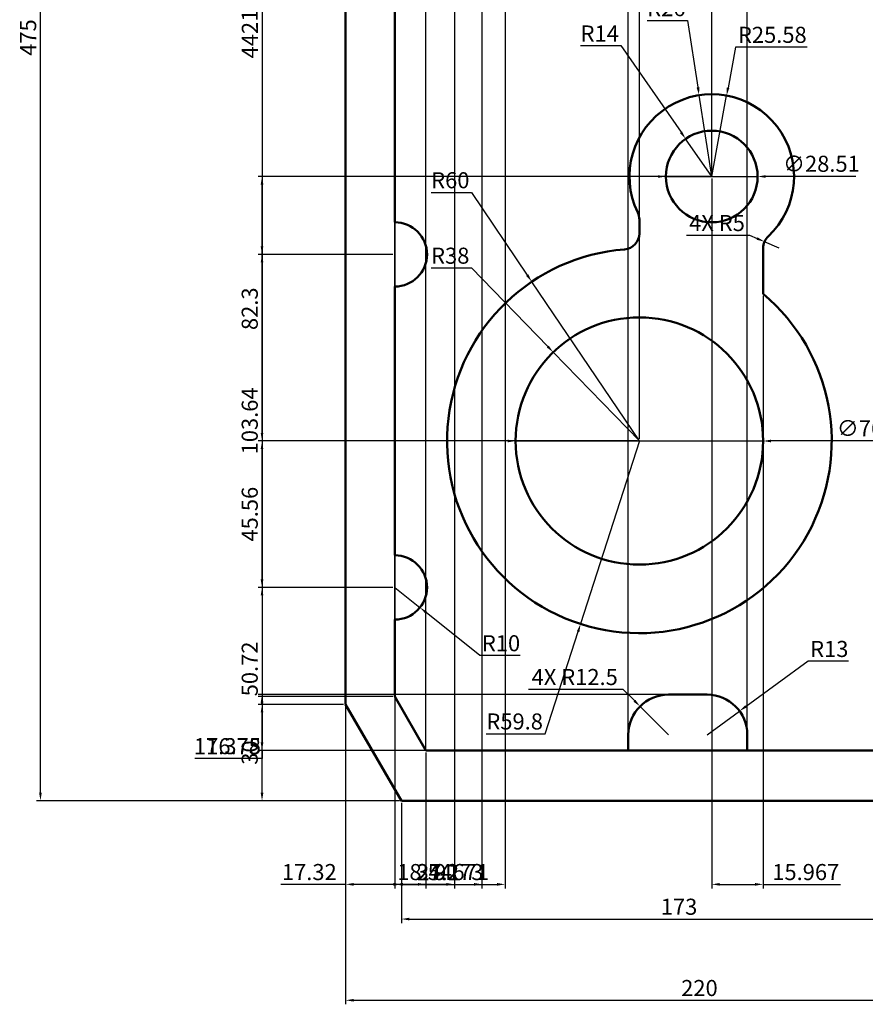
# Model space of a CAD drawing. Units: millimetres. Extents: x 1744 to 2162, y 1763 to 2334.
# Tile 1 of 5: x 1744 to 2007, y 1763 to 2070. Entities that reach past the tile are written whole.
import ezdxf

# ---------------------------------------------------------------- set-up
doc = ezdxf.new("R2010")
doc.units = ezdxf.units.MM
doc.layers.add('M-DIMS', color=2, linetype='Continuous', lineweight=25)
doc.layers.add('M-OUTL', color=7, linetype='Continuous', lineweight=50)
doc.styles.get("Standard").update_dxf_attribs({"font": 'arial.ttf'})
doc.dimstyles.new('ISO-25', dxfattribs={"dimtxt": 5, "dimasz": 2.5, "dimexe": 1.25, "dimexo": 0.625, "dimtad": 1, "dimtoh": 1, "dimdec": 0, "dimtxsty": 'Standard', "dimcen": 2.5, "dimadec": 0, "dimazin": 0, "dimtfac": 1, "dimtdec": 0, "dimtmove": 0, "dimatfit": 3, "dimfxl": 1, "dimarcsym": 0})

# ---------------------------------------------------------------- blocks, each defined once
blk = doc.blocks.new('*D1')
at = {"layer": 'Defpoints', "color": 0, "transparency": 16777216}
for p in [(1750.93, 2301.76), (1845.83, 2301.76), (1863.15, 1826.76)]:
    blk.add_point(p, dxfattribs=at)
at = {"layer": 'M-DIMS', "color": 0, "lineweight": -2, "transparency": 16777216}
for p, q in [((1845.2, 2301.76), (1749.68, 2301.76)), ((1750.93, 1829.26), (1750.93, 2299.26)), ((1862.52, 1826.76), (1749.68, 1826.76))]:
    blk.add_line(p, q, dxfattribs=at)
at = {"layer": 'M-DIMS', "color": 0, "transparency": 16777216}
for points in [[(1750.52, 2299.26), (1751.35, 2299.26), (1750.93, 2301.76)], [(1750.52, 1829.26), (1751.35, 1829.26), (1750.93, 1826.76)]]:
    blk.add_solid(points, dxfattribs=at)
at = {"layer": 'M-DIMS', "color": 0, "transparency": 16777216, "insert": (1747.76, 2064.26), "char_height": 5, "attachment_point": 5, "rotation": 90}
blk.add_mtext('475', dxfattribs=at)
blk = doc.blocks.new('*D14')
at = {"layer": 'Defpoints', "color": 0, "transparency": 16777216}
for p in [(1951.53, 2032.73), (1959.65, 2021.02)]:
    blk.add_point(p, dxfattribs=at)
at = {"layer": 'M-DIMS', "color": 0, "lineweight": -2, "transparency": 16777216}
for p, q in [((1918.86, 2061.74), (1931.41, 2061.74)), ((1931.41, 2061.74), (1950.11, 2034.78)), ((1959.65, 2021.02), (1951.53, 2032.73))]:
    blk.add_line(p, q, dxfattribs=at)
at = {"layer": 'M-DIMS', "color": 0, "transparency": 16777216}
blk.add_solid([(1950.45, 2035.02), (1949.76, 2034.55), (1951.53, 2032.73)], dxfattribs=at)
at = {"layer": 'M-DIMS', "color": 0, "transparency": 16777216, "insert": (1924.83, 2064.87), "char_height": 5, "attachment_point": 5}
blk.add_mtext('R14', dxfattribs=at)
blk = doc.blocks.new('*D15')
at = {"layer": 'Defpoints', "color": 0, "transparency": 16777216}
for p in [(1955.73, 2046.29), (1959.65, 2021.02)]:
    blk.add_point(p, dxfattribs=at)
at = {"layer": 'M-DIMS', "color": 0, "lineweight": -2, "transparency": 16777216}
for p, q in [((1939.55, 2069.57), (1952.12, 2069.57)), ((1952.12, 2069.57), (1955.35, 2048.77)), ((1959.65, 2021.02), (1955.73, 2046.29))]:
    blk.add_line(p, q, dxfattribs=at)
at = {"layer": 'M-DIMS', "color": 0, "transparency": 16777216}
blk.add_solid([(1955.76, 2048.83), (1954.94, 2048.7), (1955.73, 2046.29)], dxfattribs=at)
at = {"layer": 'M-DIMS', "color": 0, "transparency": 16777216, "insert": (1945.53, 2072.75), "char_height": 5, "attachment_point": 5}
blk.add_mtext('R26', dxfattribs=at)
blk = doc.blocks.new('*D16')
at = {"layer": 'Defpoints', "color": 0, "transparency": 16777216}
for p in [(1903.69, 1988.28), (1937.15, 1938.72)]:
    blk.add_point(p, dxfattribs=at)
at = {"layer": 'M-DIMS', "color": 0, "lineweight": -2, "transparency": 16777216}
for p, q in [((1872.4, 2016.03), (1884.96, 2016.03)), ((1884.96, 2016.03), (1902.3, 1990.35)), ((1937.15, 1938.72), (1903.69, 1988.28))]:
    blk.add_line(p, q, dxfattribs=at)
at = {"layer": 'M-DIMS', "color": 0, "transparency": 16777216}
blk.add_solid([(1902.64, 1990.58), (1901.95, 1990.12), (1903.69, 1988.28)], dxfattribs=at)
at = {"layer": 'M-DIMS', "color": 0, "transparency": 16777216, "insert": (1878.37, 2019.21), "char_height": 5, "attachment_point": 5}
blk.add_mtext('R60', dxfattribs=at)
blk = doc.blocks.new('*D17')
at = {"layer": 'Defpoints', "color": 0, "transparency": 16777216}
for p in [(1910.38, 1966.33), (1937.15, 1938.72)]:
    blk.add_point(p, dxfattribs=at)
at = {"layer": 'M-DIMS', "color": 0, "lineweight": -2, "transparency": 16777216}
for p, q in [((1872.37, 1992.55), (1884.96, 1992.55)), ((1884.96, 1992.55), (1908.64, 1968.13)), ((1937.15, 1938.72), (1910.38, 1966.33))]:
    blk.add_line(p, q, dxfattribs=at)
at = {"layer": 'M-DIMS', "color": 0, "transparency": 16777216}
blk.add_solid([(1908.93, 1968.42), (1908.34, 1967.84), (1910.38, 1966.33)], dxfattribs=at)
at = {"layer": 'M-DIMS', "color": 0, "transparency": 16777216, "insert": (1878.35, 1995.73), "char_height": 5, "attachment_point": 5}
blk.add_mtext('R38', dxfattribs=at)
blk = doc.blocks.new('*D18')
at = {"layer": 'Defpoints', "color": 0, "transparency": 16777216}
for p in [(1861.12, 1893.15), (1868.93, 1886.9)]:
    blk.add_point(p, dxfattribs=at)
at = {"layer": 'M-DIMS', "color": 0, "lineweight": -2, "transparency": 16777216}
for p, q in [((1861.12, 1893.15), (1868.93, 1886.9)), ((1887.55, 1871.97), (1870.88, 1885.33)), ((1900.1, 1871.97), (1887.55, 1871.97))]:
    blk.add_line(p, q, dxfattribs=at)
at = {"layer": 'M-DIMS', "color": 0, "transparency": 16777216}
blk.add_solid([(1871.14, 1885.66), (1870.62, 1885.01), (1868.93, 1886.9)], dxfattribs=at)
at = {"layer": 'M-DIMS', "color": 0, "transparency": 16777216, "insert": (1894.14, 1875.14), "char_height": 5, "attachment_point": 5}
blk.add_mtext('R10', dxfattribs=at)
blk = doc.blocks.new('*D19')
at = {"layer": 'Defpoints', "color": 0, "transparency": 16777216}
for p in [(1968.3, 1854.67), (1958.19, 1847.31)]:
    blk.add_point(p, dxfattribs=at)
at = {"layer": 'M-DIMS', "color": 0, "lineweight": -2, "transparency": 16777216}
for p, q in [((1989.6, 1870.18), (1970.32, 1856.14)), ((2002.17, 1870.18), (1989.6, 1870.18)), ((1958.19, 1847.31), (1968.3, 1854.67))]:
    blk.add_line(p, q, dxfattribs=at)
at = {"layer": 'M-DIMS', "color": 0, "transparency": 16777216}
blk.add_solid([(1970.08, 1856.48), (1970.57, 1855.8), (1968.3, 1854.67)], dxfattribs=at)
at = {"layer": 'M-DIMS', "color": 0, "transparency": 16777216, "insert": (1996.2, 1873.36), "char_height": 5, "attachment_point": 5}
blk.add_mtext('R13', dxfattribs=at)
blk = doc.blocks.new('*D27')
at = {"layer": 'Defpoints', "color": 0, "transparency": 16777216}
for p in [(1863.15, 1826.76), (2035.83, 1826.76), (2035.83, 1789.97)]:
    blk.add_point(p, dxfattribs=at)
at = {"layer": 'M-DIMS', "color": 0, "lineweight": -2, "transparency": 16777216}
for p, q in [((1863.15, 1826.14), (1863.15, 1788.72)), ((2035.83, 1826.14), (2035.83, 1788.72)), ((1865.65, 1789.97), (2033.33, 1789.97))]:
    blk.add_line(p, q, dxfattribs=at)
at = {"layer": 'M-DIMS', "color": 0, "transparency": 16777216}
for points in [[(1865.65, 1790.38), (1865.65, 1789.55), (1863.15, 1789.97)], [(2033.33, 1790.38), (2033.33, 1789.55), (2035.83, 1789.97)]]:
    blk.add_solid(points, dxfattribs=at)
at = {"layer": 'M-DIMS', "color": 0, "transparency": 16777216, "insert": (1949.49, 1793.15), "char_height": 5, "attachment_point": 5}
blk.add_mtext('173', dxfattribs=at)
blk = doc.blocks.new('*D28')
at = {"layer": 'Defpoints', "color": 0, "transparency": 16777216}
for p in [(1845.83, 1856.76), (2065.83, 1844.08), (2065.83, 1764.69)]:
    blk.add_point(p, dxfattribs=at)
at = {"layer": 'M-DIMS', "color": 0, "lineweight": -2, "transparency": 16777216}
for p, q in [((1845.83, 1856.14), (1845.83, 1763.44)), ((2065.83, 1843.46), (2065.83, 1763.44)), ((1848.33, 1764.69), (2063.33, 1764.69))]:
    blk.add_line(p, q, dxfattribs=at)
at = {"layer": 'M-DIMS', "color": 0, "transparency": 16777216}
for points in [[(1848.33, 1765.1), (1848.33, 1764.27), (1845.83, 1764.69)], [(2063.33, 1765.1), (2063.33, 1764.27), (2065.83, 1764.69)]]:
    blk.add_solid(points, dxfattribs=at)
at = {"layer": 'M-DIMS', "color": 0, "transparency": 16777216, "insert": (1955.83, 1767.86), "char_height": 5, "attachment_point": 5}
blk.add_mtext('220', dxfattribs=at)
blk = doc.blocks.new('*D29')
at = {"layer": 'Defpoints', "color": 0, "transparency": 16777216}
for p in [(2052.51, 2327.76), (2052.51, 1966.98), (1937.15, 1938.72)]:
    blk.add_point(p, dxfattribs=at)
at = {"layer": 'M-DIMS', "color": 0, "lineweight": -2, "transparency": 16777216}
for p, q in [((1937.15, 1939.34), (1937.15, 2329.01)), ((2052.51, 1967.6), (2052.51, 2329.01)), ((1939.65, 2327.76), (2050.01, 2327.76))]:
    blk.add_line(p, q, dxfattribs=at)
at = {"layer": 'M-DIMS', "color": 0, "transparency": 16777216}
for points in [[(1939.65, 2328.18), (1939.65, 2327.34), (1937.15, 2327.76)], [(2050.01, 2328.18), (2050.01, 2327.34), (2052.51, 2327.76)]]:
    blk.add_solid(points, dxfattribs=at)
at = {"layer": 'M-DIMS', "color": 0, "transparency": 16777216, "insert": (1994.83, 2330.94), "char_height": 5, "attachment_point": 5}
blk.add_mtext('115.35', dxfattribs=at)
blk = doc.blocks.new('*D30')
at = {"layer": 'Defpoints', "color": 0, "transparency": 16777216}
for p in [(1959.65, 2327.76), (1959.65, 2021.02), (1937.15, 1938.72)]:
    blk.add_point(p, dxfattribs=at)
at = {"layer": 'M-DIMS', "color": 0, "lineweight": -2, "transparency": 16777216}
for p, q in [((1937.15, 1939.34), (1937.15, 2329.01)), ((1959.65, 2021.64), (1959.65, 2329.01)), ((1939.65, 2327.76), (1957.15, 2327.76))]:
    blk.add_line(p, q, dxfattribs=at)
at = {"layer": 'M-DIMS', "color": 0, "transparency": 16777216}
for points in [[(1939.65, 2328.18), (1939.65, 2327.34), (1937.15, 2327.76)], [(1957.15, 2328.18), (1957.15, 2327.34), (1959.65, 2327.76)]]:
    blk.add_solid(points, dxfattribs=at)
at = {"layer": 'M-DIMS', "color": 0, "transparency": 16777216, "insert": (1948.4, 2330.94), "char_height": 5, "attachment_point": 5}
blk.add_mtext('22.5', dxfattribs=at)
blk = doc.blocks.new('*D31')
at = {"layer": 'Defpoints', "color": 0, "transparency": 16777216}
for p in [(1819.83, 1938.72), (1937.15, 1938.72), (1861.12, 1893.15)]:
    blk.add_point(p, dxfattribs=at)
at = {"layer": 'M-DIMS', "color": 0, "lineweight": -2, "transparency": 16777216}
for p, q in [((1936.53, 1938.72), (1818.58, 1938.72)), ((1819.83, 1895.65), (1819.83, 1936.22)), ((1860.5, 1893.15), (1818.58, 1893.15))]:
    blk.add_line(p, q, dxfattribs=at)
at = {"layer": 'M-DIMS', "color": 0, "transparency": 16777216}
for points in [[(1819.41, 1936.22), (1820.24, 1936.22), (1819.83, 1938.72)], [(1819.41, 1895.65), (1820.24, 1895.65), (1819.83, 1893.15)]]:
    blk.add_solid(points, dxfattribs=at)
at = {"layer": 'M-DIMS', "color": 0, "transparency": 16777216, "insert": (1816.65, 1915.94), "char_height": 5, "attachment_point": 5, "rotation": 90}
blk.add_mtext('45.56', dxfattribs=at)
blk = doc.blocks.new('*D32')
at = {"layer": 'Defpoints', "color": 0, "transparency": 16777216}
for p in [(1819.83, 2021.02), (1959.65, 2021.02), (1937.15, 1938.72)]:
    blk.add_point(p, dxfattribs=at)
at = {"layer": 'M-DIMS', "color": 0, "lineweight": -2, "transparency": 16777216}
for p, q in [((1959.03, 2021.02), (1818.58, 2021.02)), ((1819.83, 1941.22), (1819.83, 2018.52)), ((1936.53, 1938.72), (1818.58, 1938.72))]:
    blk.add_line(p, q, dxfattribs=at)
at = {"layer": 'M-DIMS', "color": 0, "transparency": 16777216}
for points in [[(1819.41, 2018.52), (1820.24, 2018.52), (1819.83, 2021.02)], [(1819.41, 1941.22), (1820.24, 1941.22), (1819.83, 1938.72)]]:
    blk.add_solid(points, dxfattribs=at)
at = {"layer": 'M-DIMS', "color": 0, "transparency": 16777216, "insert": (1816.65, 1979.87), "char_height": 5, "attachment_point": 5, "rotation": 90}
blk.add_mtext('82.3', dxfattribs=at)
blk = doc.blocks.new('*D37')
at = {"layer": 'Defpoints', "color": 0, "transparency": 16777216}
for p in [(1861.12, 2162.45), (1888.22, 2139.61), (1888.22, 1800.76)]:
    blk.add_point(p, dxfattribs=at)
at = {"layer": 'M-DIMS', "color": 0, "lineweight": -2, "transparency": 16777216}
for p, q in [((1861.12, 2161.83), (1861.12, 1799.51)), ((1888.22, 2138.98), (1888.22, 1799.51)), ((1863.62, 1800.76), (1885.72, 1800.76))]:
    blk.add_line(p, q, dxfattribs=at)
at = {"layer": 'M-DIMS', "color": 0, "transparency": 16777216}
for points in [[(1863.62, 1801.18), (1863.62, 1800.34), (1861.12, 1800.76)], [(1885.72, 1801.18), (1885.72, 1800.34), (1888.22, 1800.76)]]:
    blk.add_solid(points, dxfattribs=at)
at = {"layer": 'M-DIMS', "color": 0, "transparency": 16777216, "insert": (1874.67, 1803.9), "char_height": 5, "attachment_point": 5}
blk.add_mtext('27.1', dxfattribs=at)
blk = doc.blocks.new('*D46')
at = {"layer": 'Defpoints', "color": 0, "transparency": 16777216}
for p in [(2052.51, 2327.76), (1861.12, 1859.18), (2052.51, 1857.29)]:
    blk.add_point(p, dxfattribs=at)
at = {"layer": 'M-DIMS', "color": 0, "lineweight": -2, "transparency": 16777216}
for p, q in [((1861.12, 1859.81), (1861.12, 2329.01)), ((2052.51, 1857.91), (2052.51, 2329.01)), ((1863.62, 2327.76), (2050.01, 2327.76))]:
    blk.add_line(p, q, dxfattribs=at)
at = {"layer": 'M-DIMS', "color": 0, "transparency": 16777216}
for points in [[(1863.62, 2328.18), (1863.62, 2327.34), (1861.12, 2327.76)], [(2050.01, 2328.18), (2050.01, 2327.34), (2052.51, 2327.76)]]:
    blk.add_solid(points, dxfattribs=at)
at = {"layer": 'M-DIMS', "color": 0, "transparency": 16777216, "insert": (1956.82, 2330.94), "char_height": 5, "attachment_point": 5}
blk.add_mtext('191.4', dxfattribs=at)
blk = doc.blocks.new('*D47')
at = {"layer": 'Defpoints', "color": 0, "transparency": 16777216}
for p in [(1871.12, 2284.44), (1819.83, 1842.43), (1870.79, 1842.43)]:
    blk.add_point(p, dxfattribs=at)
at = {"layer": 'M-DIMS', "color": 0, "lineweight": -2, "transparency": 16777216}
for p, q in [((1870.5, 2284.44), (1818.58, 2284.44)), ((1819.83, 2281.94), (1819.83, 1844.93)), ((1870.17, 1842.43), (1818.58, 1842.43))]:
    blk.add_line(p, q, dxfattribs=at)
at = {"layer": 'M-DIMS', "color": 0, "transparency": 16777216}
for points in [[(1819.41, 2281.94), (1820.24, 2281.94), (1819.83, 2284.44)], [(1819.41, 1844.93), (1820.24, 1844.93), (1819.83, 1842.43)]]:
    blk.add_solid(points, dxfattribs=at)
at = {"layer": 'M-DIMS', "color": 0, "transparency": 16777216, "insert": (1816.69, 2063.44), "char_height": 5, "attachment_point": 5, "rotation": 90}
blk.add_mtext('442', dxfattribs=at)
blk = doc.blocks.new('*D48')
at = {"layer": 'Defpoints', "color": 0, "transparency": 16777216}
for p in [(1861.12, 2327.76), (1845.83, 1856.76), (1861.12, 1859.18)]:
    blk.add_point(p, dxfattribs=at)
at = {"layer": 'M-DIMS', "color": 0, "lineweight": -2, "transparency": 16777216}
for p, q in [((1845.83, 1857.39), (1845.83, 2329.01)), ((1861.12, 1859.81), (1861.12, 2329.01)), ((1848.33, 2327.76), (1858.62, 2327.76)), ((1861.12, 2327.76), (1885.17, 2327.76))]:
    blk.add_line(p, q, dxfattribs=at)
at = {"layer": 'M-DIMS', "color": 0, "transparency": 16777216}
for points in [[(1848.33, 2328.18), (1848.33, 2327.34), (1845.83, 2327.76)], [(1858.62, 2328.18), (1858.62, 2327.34), (1861.12, 2327.76)]]:
    blk.add_solid(points, dxfattribs=at)
at = {"layer": 'M-DIMS', "color": 0, "transparency": 16777216, "insert": (1874.4, 2330.94), "char_height": 5, "attachment_point": 5}
blk.add_mtext('15.298', dxfattribs=at)
blk = doc.blocks.new('*D49')
at = {"layer": 'Defpoints', "color": 0, "transparency": 16777216}
for p in [(1870.79, 1842.43), (1863.15, 1826.76), (2091.83, 1826.76)]:
    blk.add_point(p, dxfattribs=at)
at = {"layer": 'M-DIMS', "color": 0, "lineweight": -2, "transparency": 16777216}
for p, q in [((1871.42, 1842.43), (2093.08, 1842.43)), ((2091.83, 1839.93), (2091.83, 1829.26)), ((1863.77, 1826.76), (2093.08, 1826.76)), ((2091.83, 1826.76), (2091.83, 1824.26)), ((2091.83, 1824.26), (2070.91, 1824.26))]:
    blk.add_line(p, q, dxfattribs=at)
at = {"layer": 'M-DIMS', "color": 0, "transparency": 16777216}
for points in [[(2091.41, 1839.93), (2092.24, 1839.93), (2091.83, 1842.43)], [(2091.41, 1829.26), (2092.24, 1829.26), (2091.83, 1826.76)]]:
    blk.add_solid(points, dxfattribs=at)
at = {"layer": 'M-DIMS', "color": 0, "transparency": 16777216, "insert": (2081.06, 1827.44), "char_height": 5, "attachment_point": 5}
blk.add_mtext('15.673', dxfattribs=at)
blk = doc.blocks.new('*D53')
at = {"layer": 'Defpoints', "color": 0, "transparency": 16777216}
for p in [(1861.12, 2162.45), (1819.83, 1996.79), (1861.12, 1996.79)]:
    blk.add_point(p, dxfattribs=at)
at = {"layer": 'M-DIMS', "color": 0, "lineweight": -2, "transparency": 16777216}
for p, q in [((1860.5, 2162.45), (1818.58, 2162.45)), ((1819.83, 2159.95), (1819.83, 1999.29)), ((1860.5, 1996.79), (1818.58, 1996.79))]:
    blk.add_line(p, q, dxfattribs=at)
at = {"layer": 'M-DIMS', "color": 0, "transparency": 16777216}
for points in [[(1819.41, 2159.95), (1820.24, 2159.95), (1819.83, 2162.45)], [(1819.41, 1999.29), (1820.24, 1999.29), (1819.83, 1996.79)]]:
    blk.add_solid(points, dxfattribs=at)
at = {"layer": 'M-DIMS', "color": 0, "transparency": 16777216, "insert": (1816.65, 2079.62), "char_height": 5, "attachment_point": 5, "rotation": 90}
blk.add_mtext('165.66', dxfattribs=at)
blk = doc.blocks.new('*D54')
at = {"layer": 'Defpoints', "color": 0, "transparency": 16777216}
for p in [(1861.12, 1996.79), (1819.83, 1893.15), (1861.12, 1893.15)]:
    blk.add_point(p, dxfattribs=at)
at = {"layer": 'M-DIMS', "color": 0, "lineweight": -2, "transparency": 16777216}
for p, q in [((1860.5, 1996.79), (1818.58, 1996.79)), ((1819.83, 1994.29), (1819.83, 1895.65)), ((1860.5, 1893.15), (1818.58, 1893.15))]:
    blk.add_line(p, q, dxfattribs=at)
at = {"layer": 'M-DIMS', "color": 0, "transparency": 16777216}
for points in [[(1819.41, 1994.29), (1820.24, 1994.29), (1819.83, 1996.79)], [(1819.41, 1895.65), (1820.24, 1895.65), (1819.83, 1893.15)]]:
    blk.add_solid(points, dxfattribs=at)
at = {"layer": 'M-DIMS', "color": 0, "transparency": 16777216, "insert": (1816.65, 1944.97), "char_height": 5, "attachment_point": 5, "rotation": 90}
blk.add_mtext('103.64', dxfattribs=at)
blk = doc.blocks.new('*D55')
at = {"layer": 'Defpoints', "color": 0, "transparency": 16777216}
for p in [(1861.12, 1893.15), (1819.83, 1842.43), (1870.79, 1842.43)]:
    blk.add_point(p, dxfattribs=at)
at = {"layer": 'M-DIMS', "color": 0, "lineweight": -2, "transparency": 16777216}
for p, q in [((1860.5, 1893.15), (1818.58, 1893.15)), ((1819.83, 1890.65), (1819.83, 1844.93)), ((1870.17, 1842.43), (1818.58, 1842.43))]:
    blk.add_line(p, q, dxfattribs=at)
at = {"layer": 'M-DIMS', "color": 0, "transparency": 16777216}
for points in [[(1819.41, 1890.65), (1820.24, 1890.65), (1819.83, 1893.15)], [(1819.41, 1844.93), (1820.24, 1844.93), (1819.83, 1842.43)]]:
    blk.add_solid(points, dxfattribs=at)
at = {"layer": 'M-DIMS', "color": 0, "transparency": 16777216, "insert": (1816.65, 1867.79), "char_height": 5, "attachment_point": 5, "rotation": 90}
blk.add_mtext('50.72', dxfattribs=at)
blk = doc.blocks.new('*D58')
at = {"layer": 'Defpoints', "color": 0, "transparency": 16777216}
for p in [(1819.83, 1856.76), (1845.83, 1856.76), (1863.15, 1826.76)]:
    blk.add_point(p, dxfattribs=at)
at = {"layer": 'M-DIMS', "color": 0, "lineweight": -2, "transparency": 16777216}
for p, q in [((1845.2, 1856.76), (1818.58, 1856.76)), ((1819.83, 1829.26), (1819.83, 1854.26)), ((1862.52, 1826.76), (1818.58, 1826.76))]:
    blk.add_line(p, q, dxfattribs=at)
at = {"layer": 'M-DIMS', "color": 0, "transparency": 16777216}
for points in [[(1819.41, 1854.26), (1820.24, 1854.26), (1819.83, 1856.76)], [(1819.41, 1829.26), (1820.24, 1829.26), (1819.83, 1826.76)]]:
    blk.add_solid(points, dxfattribs=at)
at = {"layer": 'M-DIMS', "color": 0, "transparency": 16777216, "insert": (1816.65, 1841.76), "char_height": 5, "attachment_point": 5, "rotation": 90}
blk.add_mtext('30', dxfattribs=at)
blk = doc.blocks.new('*D59')
at = {"layer": 'Defpoints', "color": 0, "transparency": 16777216}
for p in [(1845.83, 1856.76), (1863.15, 1826.76), (1845.83, 1800.76)]:
    blk.add_point(p, dxfattribs=at)
at = {"layer": 'M-DIMS', "color": 0, "lineweight": -2, "transparency": 16777216}
for p, q in [((1845.83, 1856.14), (1845.83, 1799.51)), ((1863.15, 1826.14), (1863.15, 1799.51)), ((1845.83, 1800.76), (1825.72, 1800.76)), ((1860.65, 1800.76), (1848.33, 1800.76))]:
    blk.add_line(p, q, dxfattribs=at)
at = {"layer": 'M-DIMS', "color": 0, "transparency": 16777216}
for points in [[(1848.33, 1801.18), (1848.33, 1800.34), (1845.83, 1800.76)], [(1860.65, 1801.18), (1860.65, 1800.34), (1863.15, 1800.76)]]:
    blk.add_solid(points, dxfattribs=at)
at = {"layer": 'M-DIMS', "color": 0, "transparency": 16777216, "insert": (1834.53, 1803.94), "char_height": 5, "attachment_point": 5}
blk.add_mtext('17.32', dxfattribs=at)
blk = doc.blocks.new('*D60')
at = {"layer": 'Defpoints', "color": 0, "transparency": 16777216}
for p in [(1933.69, 2327.76), (1870.79, 1842.43), (1933.69, 1842.43)]:
    blk.add_point(p, dxfattribs=at)
at = {"layer": 'M-DIMS', "color": 0, "lineweight": -2, "transparency": 16777216}
for p, q in [((1870.79, 1843.06), (1870.79, 2329.01)), ((1933.69, 1843.06), (1933.69, 2329.01)), ((1873.29, 2327.76), (1931.19, 2327.76))]:
    blk.add_line(p, q, dxfattribs=at)
at = {"layer": 'M-DIMS', "color": 0, "transparency": 16777216}
for points in [[(1873.29, 2328.18), (1873.29, 2327.34), (1870.79, 2327.76)], [(1931.19, 2328.18), (1931.19, 2327.34), (1933.69, 2327.76)]]:
    blk.add_solid(points, dxfattribs=at)
at = {"layer": 'M-DIMS', "color": 0, "transparency": 16777216, "insert": (1902.24, 2330.94), "char_height": 5, "attachment_point": 5}
blk.add_mtext('62.9', dxfattribs=at)
blk = doc.blocks.new('*D61')
at = {"layer": 'Defpoints', "color": 0, "transparency": 16777216}
for p in [(1970.69, 2327.76), (1933.69, 1842.43), (1970.69, 1842.43)]:
    blk.add_point(p, dxfattribs=at)
at = {"layer": 'M-DIMS', "color": 0, "lineweight": -2, "transparency": 16777216}
for p, q in [((1933.69, 1843.06), (1933.69, 2329.01)), ((1970.69, 1843.06), (1970.69, 2329.01)), ((1936.19, 2327.76), (1968.19, 2327.76))]:
    blk.add_line(p, q, dxfattribs=at)
at = {"layer": 'M-DIMS', "color": 0, "transparency": 16777216}
for points in [[(1936.19, 2328.18), (1936.19, 2327.34), (1933.69, 2327.76)], [(1968.19, 2328.18), (1968.19, 2327.34), (1970.69, 2327.76)]]:
    blk.add_solid(points, dxfattribs=at)
at = {"layer": 'M-DIMS', "color": 0, "transparency": 16777216, "insert": (1952.19, 2330.94), "char_height": 5, "attachment_point": 5}
blk.add_mtext('37', dxfattribs=at)
blk = doc.blocks.new('*D62')
at = {"layer": 'Defpoints', "color": 0, "transparency": 16777216}
for p in [(1946.19, 1859.81), (1819.83, 1842.43), (1933.69, 1842.43)]:
    blk.add_point(p, dxfattribs=at)
at = {"layer": 'M-DIMS', "color": 0, "lineweight": -2, "transparency": 16777216}
for p, q in [((1945.57, 1859.81), (1818.58, 1859.81)), ((1819.83, 1857.31), (1819.83, 1844.93)), ((1933.07, 1842.43), (1818.58, 1842.43)), ((1819.83, 1842.43), (1819.83, 1839.93)), ((1819.83, 1839.93), (1798.9, 1839.93))]:
    blk.add_line(p, q, dxfattribs=at)
at = {"layer": 'M-DIMS', "color": 0, "transparency": 16777216}
for points in [[(1819.41, 1857.31), (1820.24, 1857.31), (1819.83, 1859.81)], [(1819.41, 1844.93), (1820.24, 1844.93), (1819.83, 1842.43)]]:
    blk.add_solid(points, dxfattribs=at)
at = {"layer": 'M-DIMS', "color": 0, "transparency": 16777216, "insert": (1809.05, 1843.11), "char_height": 5, "attachment_point": 5}
blk.add_mtext('17.378', dxfattribs=at)
blk = doc.blocks.new('*D63')
at = {"layer": 'Defpoints', "color": 0, "transparency": 16777216}
for p in [(1861.12, 1859.18), (1819.83, 1842.43), (1870.79, 1842.43)]:
    blk.add_point(p, dxfattribs=at)
at = {"layer": 'M-DIMS', "color": 0, "lineweight": -2, "transparency": 16777216}
for p, q in [((1860.5, 1859.18), (1818.58, 1859.18)), ((1819.83, 1856.68), (1819.83, 1844.93)), ((1870.17, 1842.43), (1818.58, 1842.43)), ((1819.83, 1842.43), (1819.83, 1839.93)), ((1819.83, 1839.93), (1802.76, 1839.93))]:
    blk.add_line(p, q, dxfattribs=at)
at = {"layer": 'M-DIMS', "color": 0, "transparency": 16777216}
for points in [[(1819.41, 1856.68), (1820.24, 1856.68), (1819.83, 1859.18)], [(1819.41, 1844.93), (1820.24, 1844.93), (1819.83, 1842.43)]]:
    blk.add_solid(points, dxfattribs=at)
at = {"layer": 'M-DIMS', "color": 0, "transparency": 16777216, "insert": (1810.98, 1843.11), "char_height": 5, "attachment_point": 5}
blk.add_mtext('16.75', dxfattribs=at)
blk = doc.blocks.new('*D64')
at = {"layer": 'Defpoints', "color": 0, "transparency": 16777216}
for p in [(1861.12, 1859.18), (1870.79, 1842.43), (1870.79, 1800.76)]:
    blk.add_point(p, dxfattribs=at)
at = {"layer": 'M-DIMS', "color": 0, "lineweight": -2, "transparency": 16777216}
for p, q in [((1861.12, 1858.56), (1861.12, 1799.51)), ((1870.79, 1841.81), (1870.79, 1799.51)), ((1863.62, 1800.76), (1868.29, 1800.76)), ((1870.79, 1800.76), (1890.45, 1800.76))]:
    blk.add_line(p, q, dxfattribs=at)
at = {"layer": 'M-DIMS', "color": 0, "transparency": 16777216}
for points in [[(1863.62, 1801.18), (1863.62, 1800.34), (1861.12, 1800.76)], [(1868.29, 1801.18), (1868.29, 1800.34), (1870.79, 1800.76)]]:
    blk.add_solid(points, dxfattribs=at)
at = {"layer": 'M-DIMS', "color": 0, "transparency": 16777216, "insert": (1881.87, 1803.94), "char_height": 5, "attachment_point": 5}
blk.add_mtext('9.671', dxfattribs=at)
blk = doc.blocks.new('*D67')
at = {"layer": 'Defpoints', "color": 0, "transparency": 16777216}
for p in [(1861.12, 2162.45), (1895.4, 2111.36), (1895.4, 1800.76)]:
    blk.add_point(p, dxfattribs=at)
at = {"layer": 'M-DIMS', "color": 0, "lineweight": -2, "transparency": 16777216}
for p, q in [((1861.12, 2161.83), (1861.12, 1799.51)), ((1895.4, 2110.73), (1895.4, 1799.51)), ((1863.62, 1800.76), (1892.9, 1800.76))]:
    blk.add_line(p, q, dxfattribs=at)
at = {"layer": 'M-DIMS', "color": 0, "transparency": 16777216}
for points in [[(1863.62, 1801.18), (1863.62, 1800.34), (1861.12, 1800.76)], [(1892.9, 1801.18), (1892.9, 1800.34), (1895.4, 1800.76)]]:
    blk.add_solid(points, dxfattribs=at)
at = {"layer": 'M-DIMS', "color": 0, "transparency": 16777216, "insert": (1878.26, 1803.94), "char_height": 5, "attachment_point": 5}
blk.add_mtext('34.273', dxfattribs=at)
blk = doc.blocks.new('*D69')
at = {"layer": 'Defpoints', "color": 0, "transparency": 16777216}
for p in [(1861.12, 2162.45), (1879.67, 2085.81), (1861.12, 1800.76)]:
    blk.add_point(p, dxfattribs=at)
at = {"layer": 'M-DIMS', "color": 0, "lineweight": -2, "transparency": 16777216}
for p, q in [((1861.12, 2161.83), (1861.12, 1799.51)), ((1879.67, 2085.19), (1879.67, 1799.51)), ((1877.17, 1800.76), (1863.62, 1800.76))]:
    blk.add_line(p, q, dxfattribs=at)
at = {"layer": 'M-DIMS', "color": 0, "transparency": 16777216}
for points in [[(1863.62, 1801.18), (1863.62, 1800.34), (1861.12, 1800.76)], [(1877.17, 1801.18), (1877.17, 1800.34), (1879.67, 1800.76)]]:
    blk.add_solid(points, dxfattribs=at)
at = {"layer": 'M-DIMS', "color": 0, "transparency": 16777216, "insert": (1870.39, 1803.94), "char_height": 5, "attachment_point": 5}
blk.add_mtext('18.54', dxfattribs=at)
blk = doc.blocks.new('*D71')
at = {"layer": 'Defpoints', "color": 0, "transparency": 16777216}
for p in [(1959.65, 2021.02), (1975.62, 1984.5), (1975.62, 1800.76)]:
    blk.add_point(p, dxfattribs=at)
at = {"layer": 'M-DIMS', "color": 0, "lineweight": -2, "transparency": 16777216}
for p, q in [((1959.65, 2020.39), (1959.65, 1799.51)), ((1975.62, 1983.88), (1975.62, 1799.51)), ((1962.15, 1800.76), (1973.12, 1800.76)), ((1975.62, 1800.76), (1999.66, 1800.76))]:
    blk.add_line(p, q, dxfattribs=at)
at = {"layer": 'M-DIMS', "color": 0, "transparency": 16777216}
for points in [[(1962.15, 1801.18), (1962.15, 1800.34), (1959.65, 1800.76)], [(1973.12, 1801.18), (1973.12, 1800.34), (1975.62, 1800.76)]]:
    blk.add_solid(points, dxfattribs=at)
at = {"layer": 'M-DIMS', "color": 0, "transparency": 16777216, "insert": (1988.89, 1803.94), "char_height": 5, "attachment_point": 5}
blk.add_mtext('15.967', dxfattribs=at)
blk = doc.blocks.new('*D76')
at = {"layer": 'Defpoints', "color": 0, "transparency": 16777216}
for p in [(1976.03, 2000.74), (1980.62, 1998.75)]:
    blk.add_point(p, dxfattribs=at)
at = {"layer": 'M-DIMS', "color": 0, "lineweight": -2, "transparency": 16777216}
for p, q in [((1951.77, 2002.72), (1971.44, 2002.72)), ((1971.44, 2002.72), (1973.74, 2001.73)), ((1980.62, 1998.75), (1976.03, 2000.74))]:
    blk.add_line(p, q, dxfattribs=at)
at = {"layer": 'M-DIMS', "color": 0, "transparency": 16777216}
blk.add_solid([(1973.9, 2002.11), (1973.57, 2001.34), (1976.03, 2000.74)], dxfattribs=at)
at = {"layer": 'M-DIMS', "color": 0, "transparency": 16777216, "insert": (1961.29, 2005.89), "char_height": 5, "attachment_point": 5}
blk.add_mtext('4X R5', dxfattribs=at)
blk = doc.blocks.new('*D77')
at = {"layer": 'Defpoints', "color": 0, "transparency": 16777216}
for p in [(1937.15, 1938.72), (1918.87, 1881.78)]:
    blk.add_point(p, dxfattribs=at)
at = {"layer": 'M-DIMS', "color": 0, "lineweight": -2, "transparency": 16777216}
for p, q in [((1937.15, 1938.72), (1918.87, 1881.78)), ((1907.9, 1847.62), (1918.1, 1879.4)), ((1889.49, 1847.62), (1907.9, 1847.62))]:
    blk.add_line(p, q, dxfattribs=at)
at = {"layer": 'M-DIMS', "color": 0, "transparency": 16777216}
blk.add_solid([(1917.71, 1879.53), (1918.5, 1879.28), (1918.87, 1881.78)], dxfattribs=at)
at = {"layer": 'M-DIMS', "color": 0, "transparency": 16777216, "insert": (1898.38, 1850.8), "char_height": 5, "attachment_point": 5}
blk.add_mtext('R59.8', dxfattribs=at)
blk = doc.blocks.new('*D78')
at = {"layer": 'Defpoints', "color": 0, "transparency": 16777216}
for p in [(1898.69, 1938.72), (1975.62, 1938.72)]:
    blk.add_point(p, dxfattribs=at)
at = {"layer": 'M-DIMS', "color": 0, "lineweight": -2, "transparency": 16777216}
for p, q in [((1896.19, 1938.72), (1893.69, 1938.72)), ((1898.69, 1938.72), (1975.62, 1938.72)), ((1998.7, 1938.72), (1978.12, 1938.72)), ((2021.64, 1938.72), (1998.7, 1938.72))]:
    blk.add_line(p, q, dxfattribs=at)
at = {"layer": 'M-DIMS', "color": 0, "transparency": 16777216}
for points in [[(1896.19, 1939.13), (1896.19, 1938.3), (1898.69, 1938.72)], [(1978.12, 1939.13), (1978.12, 1938.3), (1975.62, 1938.72)]]:
    blk.add_solid(points, dxfattribs=at)
at = {"layer": 'M-DIMS', "color": 0, "transparency": 16777216, "insert": (2010.48, 1942.03), "char_height": 5, "attachment_point": 5}
blk.add_mtext('∅76.93', dxfattribs=at)
blk = doc.blocks.new('*D81')
at = {"layer": 'Defpoints', "color": 0, "transparency": 16777216}
for p in [(1964.27, 2046.18), (1959.65, 2021.02)]:
    blk.add_point(p, dxfattribs=at)
at = {"layer": 'M-DIMS', "color": 0, "lineweight": -2, "transparency": 16777216}
for p, q in [((1967.03, 2061.28), (1964.72, 2048.64)), ((1989.33, 2061.28), (1967.03, 2061.28)), ((1959.65, 2021.02), (1964.27, 2046.18))]:
    blk.add_line(p, q, dxfattribs=at)
at = {"layer": 'M-DIMS', "color": 0, "transparency": 16777216}
blk.add_solid([(1964.31, 2048.71), (1965.13, 2048.56), (1964.27, 2046.18)], dxfattribs=at)
at = {"layer": 'M-DIMS', "color": 0, "transparency": 16777216, "insert": (1978.49, 2064.45), "char_height": 5, "attachment_point": 5}
blk.add_mtext('R25.58', dxfattribs=at)
blk = doc.blocks.new('*D83')
at = {"layer": 'Defpoints', "color": 0, "transparency": 16777216}
for p in [(1945.4, 2021.02), (1973.91, 2021.02)]:
    blk.add_point(p, dxfattribs=at)
at = {"layer": 'M-DIMS', "color": 0, "lineweight": -2, "transparency": 16777216}
for p, q in [((1942.9, 2021.02), (1940.4, 2021.02)), ((1945.4, 2021.02), (1973.91, 2021.02)), ((1982.46, 2021.02), (1976.41, 2021.02)), ((2004.44, 2021.02), (1982.46, 2021.02))]:
    blk.add_line(p, q, dxfattribs=at)
at = {"layer": 'M-DIMS', "color": 0, "transparency": 16777216}
for points in [[(1942.9, 2021.43), (1942.9, 2020.6), (1945.4, 2021.02)], [(1976.41, 2021.43), (1976.41, 2020.6), (1973.91, 2021.02)]]:
    blk.add_solid(points, dxfattribs=at)
at = {"layer": 'M-DIMS', "color": 0, "transparency": 16777216, "insert": (1993.76, 2024.33), "char_height": 5, "attachment_point": 5}
blk.add_mtext('∅28.51', dxfattribs=at)
blk = doc.blocks.new('*D84')
at = {"layer": 'Defpoints', "color": 0, "transparency": 16777216}
for p in [(1937.36, 1856.15), (1946.19, 1847.31)]:
    blk.add_point(p, dxfattribs=at)
at = {"layer": 'M-DIMS', "color": 0, "lineweight": -2, "transparency": 16777216}
for p, q in [((1902.67, 1861.45), (1932.05, 1861.45)), ((1932.05, 1861.45), (1935.59, 1857.92)), ((1946.19, 1847.31), (1937.36, 1856.15))]:
    blk.add_line(p, q, dxfattribs=at)
at = {"layer": 'M-DIMS', "color": 0, "transparency": 16777216}
blk.add_solid([(1935.88, 1858.21), (1935.29, 1857.62), (1937.36, 1856.15)], dxfattribs=at)
at = {"layer": 'M-DIMS', "color": 0, "transparency": 16777216, "insert": (1917.05, 1864.63), "char_height": 5, "attachment_point": 5}
blk.add_mtext('4X R12.5', dxfattribs=at)

msp = doc.modelspace()

# ---------------------------------------------------------------- linework, layer by layer
at = {"layer": 'M-OUTL'}
for p, q in [((1845.8255, 2301.7604), (1845.8255, 1856.7604)), ((1861.1237, 2152.4535), (1861.1237, 2006.7886)), ((1937.1543, 2003.3225), (1937.1543, 2007.6377)), ((1975.6215, 1984.5009), (1975.6215, 1998.7536)), ((1861.1237, 1986.7886), (1861.1237, 1903.1533)), ((1861.1237, 1883.1533), (1861.1237, 1859.184)), ((1946.1942, 1859.8112), (1958.1942, 1859.8112)), ((1845.8255, 1856.7604), (1863.146, 1826.7604)), ((1861.1237, 1859.184), (1870.7949, 1842.4331)), ((1933.6942, 1847.3112), (1933.6942, 1842.4331)), ((1970.6942, 1847.3112), (1970.6942, 1842.4331)), ((1870.7949, 1842.4331), (2026.7759, 1842.4331)), ((1863.146, 1826.7604), (2035.8255, 1826.7604))]:
    msp.add_line(p, q, dxfattribs=at)
for centre, radius in [((1959.6543, 2021.0157), 14.2555), ((1959.6543, 2021.0157), 14.2555), ((1959.6543, 2021.0157), 14.2555), ((1937.1543, 1938.7171), 38.4671)]:
    msp.add_circle(centre, radius, dxfattribs=at)
for centre, radius, start, end in [((1959.6543, 2021.0157), 25.5814, 313.284158, 205.94169), ((1861.1237, 1996.7886), 10, 270, 90), ((1932.1543, 2007.6377), 5, 0, 25.94169), ((1932.1543, 2003.3225), 5, 274.425462, 0), ((1980.6215, 1998.7536), 5, 133.284158, 180), ((1937.1543, 1938.7171), 59.7987, 94.425462, 49.963353), ((1861.1237, 1893.1533), 10, 270, 90), ((1946.1942, 1847.3112), 12.5, 90, 180), ((1958.1942, 1847.3112), 12.5, 0, 90)]:
    msp.add_arc(centre, radius, start, end, dxfattribs=at)

# ---------------------------------------------------------------- dimensions: what is measured, and where the dimension line sits
at = {"layer": 'M-DIMS'}
for base, p1, p2, override, picture, middle in [((1861.1237, 2327.7604), (1845.8255, 1856.7604), (1861.1237, 1859.184), {"dimdec": 3, "dimlfac": 1, "dimrnd": 0, "dimzin": 0, "dimdsep": 46, "dimlunit": 2}, '*D48', (1874.3971, 2330.9382)), ((2052.5068, 2327.7604), (1861.1237, 1859.184), (2052.5068, 1857.2889), {"dimdec": 1, "dimlfac": 1, "dimrnd": 0, "dimzin": 0, "dimdsep": 46, "dimlunit": 2}, '*D46', (1956.8153, 2330.9382)), ((1933.6942, 2327.7604), (1870.7949, 1842.4331), (1933.6942, 1842.4331), {"dimdec": 1, "dimlfac": 1, "dimrnd": 0, "dimzin": 0, "dimdsep": 46, "dimlunit": 2}, '*D60', (1902.2445, 2330.9382)), ((1970.6942, 2327.7604), (1933.6942, 1842.4331), (1970.6942, 1842.4331), {"dimdec": 0, "dimlfac": 1, "dimrnd": 0, "dimzin": 0, "dimdsep": 46, "dimlunit": 2}, '*D61', (1952.1942, 2330.9399)), ((2052.5068, 2327.7604), (1937.1543, 1938.7171), (2052.5068, 1966.9753), {"dimdec": 2, "dimlfac": 1, "dimrnd": 0, "dimzin": 0, "dimdsep": 46, "dimlunit": 2}, '*D29', (1994.8306, 2330.9399)), ((1959.6543, 2327.7604), (1937.1543, 1938.7171), (1959.6543, 2021.0157), {"dimdec": 1, "dimlfac": 1, "dimrnd": 0, "dimzin": 0, "dimdsep": 46, "dimlunit": 2}, '*D30', (1948.4043, 2330.9382)), ((1888.2243, 1800.7604), (1861.1237, 2162.4535), (1888.2243, 2139.6094), {"dimdec": 1, "dimlfac": 1, "dimrnd": 0, "dimzin": 0, "dimdsep": 46, "dimlunit": 2}, '*D37', (1874.674, 1803.8956)), ((1895.39722, 1800.76037), (1861.12374, 2162.45354), (1895.39722, 2111.35824), {"dimdec": 3, "dimlfac": 1, "dimrnd": 0, "dimzin": 0, "dimdsep": 46, "dimlunit": 2}, '*D67', (1878.26048, 1803.93994)), ((1861.1237, 1800.7604), (1879.6653, 2085.814), (1861.1237, 2162.4535), {"dimdec": 2, "dimlfac": 1, "dimrnd": 0, "dimzin": 0, "dimdsep": 46, "dimlunit": 2}, '*D69', (1870.3945, 1803.9382)), ((1975.6215, 1800.7604), (1959.6543, 2021.0157), (1975.6215, 1984.5009), {"dimdec": 3, "dimlfac": 1, "dimrnd": 0, "dimzin": 0, "dimdsep": 46, "dimlunit": 2}, '*D71', (1988.8897, 1803.9382)), ((1845.8255, 1800.7604), (1863.146, 1826.7604), (1845.8255, 1856.7604), {"dimdec": 2, "dimlfac": 1, "dimrnd": 0, "dimzin": 0, "dimdsep": 46, "dimlunit": 2}, '*D59', (1834.5252, 1803.9399)), ((2065.8255, 1764.685), (1845.8255, 1856.7604), (2065.8255, 1844.0809), {"dimclrd": 0, "dimclre": 0, "dimclrt": 0}, '*D28', (1955.8255, 1767.8629)), ((1870.7949, 1800.7604), (1861.1237, 1859.184), (1870.7949, 1842.4331), {"dimdec": 3, "dimlfac": 1, "dimrnd": 0, "dimzin": 0, "dimdsep": 46, "dimlunit": 2}, '*D64', (1881.8735, 1803.9382)), ((2035.8255, 1789.9672), (1863.146, 1826.7604), (2035.8255, 1826.7604), {"dimclrd": 0, "dimclre": 0, "dimclrt": 0}, '*D27', (1949.4857, 1793.1468))]:
    dim = msp.add_linear_dim(base=base, p1=p1, p2=p2, dimstyle='ISO-25', override=override, dxfattribs=at)
    dim.commit()
    dim.dimension.update_dxf_attribs({"geometry": picture, "text_midpoint": middle})
for base, p1, p2, override, picture, middle in [((1750.9321, 2301.7604), (1863.146, 1826.7604), (1845.8255, 2301.7604), {"dimclrd": 0, "dimclre": 0, "dimclrt": 0}, '*D1', (1747.7645, 2064.2604)), ((1819.8255, 1842.4331), (1871.1237, 2284.4372), (1870.7949, 1842.4331), {"dimdec": 0, "dimlfac": 1, "dimrnd": 0, "dimzin": 0, "dimdsep": 46, "dimlunit": 2}, '*D47', (1816.6902, 2063.4352)), ((1819.8255, 1996.7886), (1861.1237, 2162.4535), (1861.1237, 1996.7886), {"dimdec": 2, "dimlfac": 1, "dimrnd": 0, "dimzin": 0, "dimdsep": 46, "dimlunit": 2}, '*D53', (1816.6476, 2079.621)), ((1819.8255, 2021.0157), (1937.1543, 1938.7171), (1959.6543, 2021.0157), {"dimdec": 1, "dimlfac": 1, "dimrnd": 0, "dimzin": 0, "dimdsep": 46, "dimlunit": 2}, '*D32', (1816.6459, 1979.8664)), ((1819.8255, 1893.1533), (1861.1237, 1996.7886), (1861.1237, 1893.1533), {"dimdec": 2, "dimlfac": 1, "dimrnd": 0, "dimzin": 0, "dimdsep": 46, "dimlunit": 2}, '*D54', (1816.6459, 1944.9709)), ((1819.8255, 1938.7171), (1861.1237, 1893.1533), (1937.1543, 1938.7171), {"dimdec": 2, "dimlfac": 1, "dimrnd": 0, "dimzin": 0, "dimdsep": 46, "dimlunit": 2}, '*D31', (1816.6476, 1915.9352)), ((1819.8255, 1842.4331), (1861.1237, 1893.1533), (1870.7949, 1842.4331), {"dimdec": 2, "dimlfac": 1, "dimrnd": 0, "dimzin": 0, "dimdsep": 46, "dimlunit": 2}, '*D55', (1816.6476, 1867.7932)), ((1819.8255, 1842.4331), (1946.1942, 1859.8112), (1933.6942, 1842.4331), {"dimdec": 3, "dimlfac": 1, "dimrnd": 0, "dimzin": 0, "dimdsep": 46, "dimlunit": 2}, '*D62', (1809.0521, 1843.1127)), ((1819.8255, 1842.4331), (1861.1237, 1859.184), (1870.7949, 1842.4331), {"dimdec": 2, "dimlfac": 1, "dimrnd": 0, "dimzin": 0, "dimdsep": 46, "dimlunit": 2}, '*D63', (1810.9808, 1843.111)), ((1819.8255, 1856.7604), (1863.146, 1826.7604), (1845.8255, 1856.7604), {"dimdec": 0, "dimlfac": 1, "dimrnd": 0, "dimzin": 0, "dimdsep": 46, "dimlunit": 2}, '*D58', (1816.6459, 1841.7604)), ((2091.8255, 1826.7604), (1870.7949, 1842.4331), (1863.146, 1826.7604), {"dimdec": 3, "dimlfac": 1, "dimrnd": 0, "dimzin": 0, "dimdsep": 46, "dimlunit": 2}, '*D49', (2081.0572, 1827.4399))]:
    dim = msp.add_linear_dim(base=base, p1=p1, p2=p2, angle=90, dimstyle='ISO-25', override=override, dxfattribs=at)
    dim.commit()
    dim.dimension.update_dxf_attribs({"geometry": picture, "text_midpoint": middle})
for center, mpoint, override, picture, middle in [((1959.6543, 2021.0157), (1955.7334, 2046.2948), {"dimclrd": 0, "dimclre": 0, "dimclrt": 0}, '*D15', (1945.5266, 2069.568)), ((1959.6543, 2021.0157), (1951.531, 2032.7302), {"dimclrd": 0, "dimclre": 0, "dimclrt": 0}, '*D14', (1924.8264, 2061.7391)), ((1959.6543, 2021.0157), (1964.267, 2046.1778), {"dimdec": 2, "dimlfac": 1, "dimrnd": 0, "dimzin": 0, "dimdsep": 46, "dimlunit": 2}, '*D81', (1978.4934, 2061.2751)), ((1937.1543, 1938.7171), (1903.6946, 1988.2784), {"dimclrd": 0, "dimclre": 0, "dimclrt": 0}, '*D16', (1878.3668, 2016.0328)), ((1937.1543, 1938.7171), (1910.3758, 1966.3328), {"dimclrd": 0, "dimclre": 0, "dimclrt": 0}, '*D17', (1878.3532, 1992.5461)), ((1937.1543, 1938.7171), (1918.8689, 1881.7827), {"dimdec": 1, "dimlfac": 1, "dimrnd": 0, "dimzin": 0, "dimdsep": 46, "dimlunit": 2}, '*D77', (1898.3811, 1847.6221)), ((1861.1237, 1893.1533), (1868.9253, 1886.8974), {"dimclrd": 0, "dimclre": 0, "dimclrt": 0}, '*D18', (1894.1374, 1871.965)), ((1958.1942, 1847.3112), (1968.2996, 1854.6685), {"dimclrd": 0, "dimclre": 0, "dimclrt": 0}, '*D19', (1996.1985, 1870.1762))]:
    dim = msp.add_radius_dim(center=center, mpoint=mpoint, dimstyle='ISO-25', override=override, dxfattribs=at)
    dim.commit()
    dim.dimension.update_dxf_attribs({"geometry": picture, "text_midpoint": middle, "dimtype": 164})
for p1, p2, picture, middle in [((1945.3989, 2021.0155), (1973.9098, 2021.016), '*D83', (1982.4631, 2021.0162)), ((1898.6872, 1938.7172), (1975.6215, 1938.717), '*D78', (1998.7017, 1938.717))]:
    dim = msp.add_diameter_dim_2p(p1=p1, p2=p2, dimstyle='ISO-25', override={"dimdec": 2, "dimlfac": 1, "dimrnd": 0, "dimzin": 0, "dimdsep": 46, "dimlunit": 2}, dxfattribs=at)
    dim.commit()
    dim.dimension.update_dxf_attribs({"geometry": picture, "text_midpoint": middle, "dimtype": 163})
dim = msp.add_radius_dim(center=(1980.6215, 1998.7536), mpoint=(1976.0312, 2000.7359), text='4X <>', dimstyle='ISO-25', override={"dimdec": 0, "dimlfac": 1, "dimrnd": 0, "dimzin": 0, "dimdsep": 46, "dimlunit": 2}, dxfattribs=at)
dim.commit()
dim.dimension.update_dxf_attribs({"geometry": '*D76', "text_midpoint": (1961.2934, 2005.8858)})
dim = msp.add_radius_dim(center=(1946.1942, 1847.3112), mpoint=(1937.3552, 1856.1498), text='4X <>', dimstyle='ISO-25', override={"dimdec": 1, "dimlfac": 1, "dimrnd": 0, "dimzin": 0, "dimdsep": 46, "dimlunit": 2}, dxfattribs=at)
dim.commit()
dim.dimension.update_dxf_attribs({"geometry": '*D84', "text_midpoint": (1917.0492, 1861.453), "dimtype": 164})

doc.saveas('drawing.dxf')
